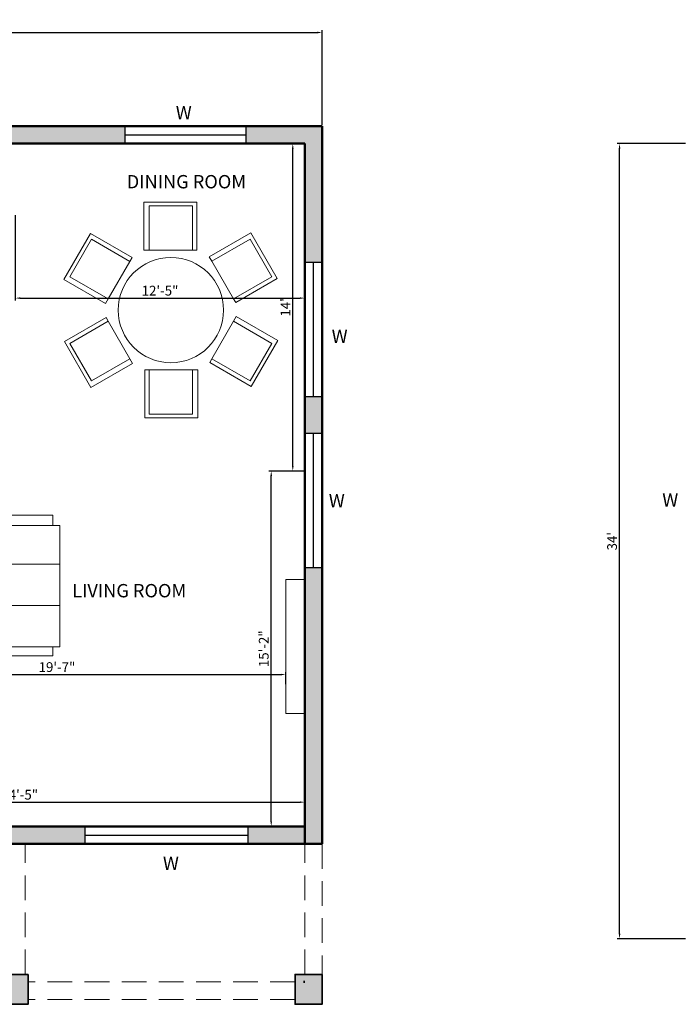
# Model space of a CAD drawing. Units: inches. Extents: x 1838 to 3464, y 573 to 2547.
# Tile 3 of 6: x 2449 to 2788, y 1302 to 1808. Entities that reach past the tile are written whole.
import ezdxf

# ---------------------------------------------------------------- set-up
doc = ezdxf.new("R2010")
doc.units = ezdxf.units.IN
doc.linetypes.add('DASHED', pattern=[19.05, 12.7, -6.35])
for name, color, linetype, lineweight in [('A-ANNO-DIMS', 2, 'Continuous', 18), ('A-ANNO-TEXT', 7, 'Continuous', 18), ('A-AREA-IDEN', 3, 'Continuous', 18), ('A-COLS', 6, 'Continuous', 35), ('A-FLOR-OVHD', 8, 'DASHED', 18), ('A-FURN', 8, 'Continuous', 18), ('A-GLAZ', 3, 'Continuous', 25), ('A-WALL', 1, 'Continuous', 50), ('A-WALL-PATT', 8, 'Continuous', 13)]:
    doc.layers.add(name, color=color, linetype=linetype, lineweight=lineweight)
doc.styles.get("Standard").update_dxf_attribs({"font": 'arial.ttf'})
doc.dimstyles.new('ISO-25', dxfattribs={"dimtxt": 5, "dimasz": 2.5, "dimexe": 1.25, "dimexo": 0.625, "dimtad": 1, "dimdec": 0, "dimlunit": 4, "dimtxsty": 'Standard', "dimcen": 2.5, "dimadec": 0, "dimazin": 0, "dimtfac": 1, "dimtdec": 0, "dimtmove": 0, "dimatfit": 3, "dimfxl": 1, "dimarcsym": 0})

# ---------------------------------------------------------------- blocks, each defined once
blk = doc.blocks.new('*U5')
for p, q in [((-13.85, 16.56), (-13.85, 41.18)), ((-13.85, 41.18), (13.34, 41.18)), ((13.34, 41.18), (13.34, 16.56)), ((-11.15, 16.56), (-13.85, 16.56)), ((13.34, 16.56), (11.13, 16.56))]:
    blk.add_line(p, q)
blk.add_lwpolyline([(-11.15, 16.56), (11.13, 16.56), (11.13, 39.27), (-11.15, 39.27)], close=True)
blk.add_circle((0, -14.18), 27.01)
blk = doc.blocks.new('*U6')
at = {"layer": 'A-FURN', "transparency": 16777216}
blk.add_blockref('*U5', (2526.78, 1672.86), dxfattribs=at)
for p, rotation in [((2514.5, 1665.77), 60), ((2539.06, 1665.77), 300), ((2514.5, 1651.59), 120), ((2539.06, 1651.59), 240), ((2526.78, 1644.5), 180)]:
    blk.add_blockref('*U5', p, dxfattribs=dict(at, rotation=rotation))
blk = doc.blocks.new('*D13')
at = {"layer": 'A-ANNO-DIMS', "color": 0, "lineweight": -2, "transparency": 16777216}
for p, q in [((2302.96, 1394.32), (2302.96, 1407.41)), ((2305.46, 1406.16), (2592.96, 1406.16)), ((2595.46, 1394.32), (2595.46, 1407.41))]:
    blk.add_line(p, q, dxfattribs=at)
at = {"layer": 'A-ANNO-DIMS', "color": 0, "lineweight": 100, "transparency": 16777216}
for points in [[(2305.46, 1406.58), (2305.46, 1405.75), (2302.96, 1406.16)], [(2592.96, 1406.58), (2592.96, 1405.75), (2595.46, 1406.16)]]:
    blk.add_solid(points, dxfattribs=at)
at = {"layer": 'Defpoints', "color": 0, "lineweight": 100, "transparency": 16777216}
for p in [(2595.46, 1406.16), (2302.96, 1393.69), (2595.46, 1393.69)]:
    blk.add_point(p, dxfattribs=at)
at = {"layer": 'A-ANNO-DIMS', "color": 0, "transparency": 16777216, "insert": (2449.21, 1409.34), "char_height": 5, "attachment_point": 5}
blk.add_mtext('24\'-5"', dxfattribs=at)
blk = doc.blocks.new('*D14')
at = {"layer": 'A-ANNO-DIMS', "color": 0, "lineweight": -2, "transparency": 16777216}
for p, q in [((2594.83, 1576.09), (2577.01, 1576.09)), ((2578.26, 1396.19), (2578.26, 1573.59)), ((2594.83, 1393.69), (2577.01, 1393.69))]:
    blk.add_line(p, q, dxfattribs=at)
at = {"layer": 'A-ANNO-DIMS', "color": 0, "lineweight": 100, "transparency": 16777216}
for points in [[(2577.85, 1573.59), (2578.68, 1573.59), (2578.26, 1576.09)], [(2577.85, 1396.19), (2578.68, 1396.19), (2578.26, 1393.69)]]:
    blk.add_solid(points, dxfattribs=at)
at = {"layer": 'Defpoints', "color": 0, "lineweight": 100, "transparency": 16777216}
for p in [(2578.26, 1576.09), (2595.46, 1576.09), (2595.46, 1393.69)]:
    blk.add_point(p, dxfattribs=at)
at = {"layer": 'A-ANNO-DIMS', "color": 0, "transparency": 16777216, "insert": (2575.08, 1484.89), "char_height": 5, "attachment_point": 5, "rotation": 90}
blk.add_mtext('15\'-2"', dxfattribs=at)
blk = doc.blocks.new('*D15')
at = {"layer": 'A-ANNO-DIMS', "color": 0, "lineweight": -2, "transparency": 16777216}
for p, q in [((2594.83, 1744.09), (2588.08, 1744.09)), ((2589.33, 1578.59), (2589.33, 1741.59)), ((2594.83, 1576.09), (2588.08, 1576.09))]:
    blk.add_line(p, q, dxfattribs=at)
at = {"layer": 'A-ANNO-DIMS', "color": 0, "lineweight": 100, "transparency": 16777216}
for points in [[(2588.91, 1741.59), (2589.74, 1741.59), (2589.33, 1744.09)], [(2588.91, 1578.59), (2589.74, 1578.59), (2589.33, 1576.09)]]:
    blk.add_solid(points, dxfattribs=at)
at = {"layer": 'Defpoints', "color": 0, "lineweight": 100, "transparency": 16777216}
for p in [(2589.33, 1744.09), (2595.46, 1744.09), (2595.46, 1576.09)]:
    blk.add_point(p, dxfattribs=at)
at = {"layer": 'A-ANNO-DIMS', "color": 0, "transparency": 16777216, "insert": (2586.19, 1660.09), "char_height": 5, "attachment_point": 5, "rotation": 90}
blk.add_mtext("14'", dxfattribs=at)
blk = doc.blocks.new('*D16')
at = {"layer": 'A-ANNO-DIMS', "color": 0, "lineweight": -2, "transparency": 16777216}
for p, q in [((2446.96, 1707.46), (2446.96, 1663.58)), ((2595.46, 1707.46), (2595.46, 1663.58)), ((2449.46, 1664.83), (2592.96, 1664.83))]:
    blk.add_line(p, q, dxfattribs=at)
at = {"layer": 'A-ANNO-DIMS', "color": 0, "lineweight": 100, "transparency": 16777216}
for points in [[(2449.46, 1665.25), (2449.46, 1664.41), (2446.96, 1664.83)], [(2592.96, 1665.25), (2592.96, 1664.41), (2595.46, 1664.83)]]:
    blk.add_solid(points, dxfattribs=at)
at = {"layer": 'Defpoints', "color": 0, "lineweight": 100, "transparency": 16777216}
for p in [(2446.96, 1708.09), (2595.46, 1708.09), (2595.46, 1664.83)]:
    blk.add_point(p, dxfattribs=at)
at = {"layer": 'A-ANNO-DIMS', "color": 0, "transparency": 16777216, "insert": (2521.21, 1668.01), "char_height": 5, "attachment_point": 5}
blk.add_mtext('12\'-5"', dxfattribs=at)
blk = doc.blocks.new('*D17')
at = {"layer": 'A-ANNO-DIMS', "color": 0, "lineweight": -2, "transparency": 16777216}
for p, q in [((2350.96, 1466.71), (2350.96, 1472.89)), ((2353.46, 1471.64), (2583.23, 1471.64)), ((2585.73, 1466.71), (2585.73, 1472.89))]:
    blk.add_line(p, q, dxfattribs=at)
at = {"layer": 'A-ANNO-DIMS', "color": 0, "lineweight": 100, "transparency": 16777216}
for points in [[(2353.46, 1472.06), (2353.46, 1471.23), (2350.96, 1471.64)], [(2583.23, 1472.06), (2583.23, 1471.23), (2585.73, 1471.64)]]:
    blk.add_solid(points, dxfattribs=at)
at = {"layer": 'Defpoints', "color": 0, "lineweight": 100, "transparency": 16777216}
for p in [(2585.73, 1471.64), (2350.96, 1466.09), (2585.73, 1466.09)]:
    blk.add_point(p, dxfattribs=at)
at = {"layer": 'A-ANNO-DIMS', "color": 0, "transparency": 16777216, "insert": (2468.34, 1474.82), "char_height": 5, "attachment_point": 5}
blk.add_mtext('19\'-7"', dxfattribs=at)
blk = doc.blocks.new('*D20')
at = {"layer": 'A-ANNO-DIMS', "color": 0, "lineweight": -2, "transparency": 16777216}
for p, q in [((2124.46, 1753.71), (2124.46, 1802.37)), ((2126.96, 1801.12), (2601.96, 1801.12)), ((2604.46, 1753.71), (2604.46, 1802.37))]:
    blk.add_line(p, q, dxfattribs=at)
at = {"layer": 'A-ANNO-DIMS', "color": 0, "lineweight": 100, "transparency": 16777216}
for points in [[(2126.96, 1801.54), (2126.96, 1800.7), (2124.46, 1801.12)], [(2601.96, 1801.54), (2601.96, 1800.7), (2604.46, 1801.12)]]:
    blk.add_solid(points, dxfattribs=at)
at = {"layer": 'Defpoints', "color": 0, "lineweight": 100, "transparency": 16777216}
for p in [(2604.46, 1801.12), (2124.46, 1753.09), (2604.46, 1753.09)]:
    blk.add_point(p, dxfattribs=at)
at = {"layer": 'A-ANNO-DIMS', "color": 0, "transparency": 16777216, "insert": (2364.46, 1804.3), "char_height": 5, "attachment_point": 5}
blk.add_mtext("40'", dxfattribs=at)
blk = doc.blocks.new('*D66')
at = {"layer": 'A-ANNO-DIMS', "color": 0, "lineweight": -2, "transparency": 16777216}
for p, q in [((2790.9, 1744.09), (2755.73, 1744.09)), ((2756.98, 1338.59), (2756.98, 1741.59)), ((2790.9, 1336.09), (2755.73, 1336.09))]:
    blk.add_line(p, q, dxfattribs=at)
at = {"layer": 'A-ANNO-DIMS', "color": 0, "lineweight": 100, "transparency": 16777216}
for points in [[(2756.56, 1741.59), (2757.39, 1741.59), (2756.98, 1744.09)], [(2756.56, 1338.59), (2757.39, 1338.59), (2756.98, 1336.09)]]:
    blk.add_solid(points, dxfattribs=at)
at = {"layer": 'Defpoints', "color": 0, "lineweight": 100, "transparency": 16777216}
for p in [(2756.98, 1744.09), (2791.52, 1744.09), (2791.52, 1336.09)]:
    blk.add_point(p, dxfattribs=at)
at = {"layer": 'A-ANNO-DIMS', "color": 0, "transparency": 16777216, "insert": (2753.8, 1540.09), "char_height": 5, "attachment_point": 5, "rotation": 90}
blk.add_mtext("34'", dxfattribs=at)

msp = doc.modelspace()

# ---------------------------------------------------------------- hatches: boundary and pattern name
at = {"layer": 'A-WALL-PATT'}
h = msp.add_hatch(color=256, dxfattribs=at)
h.dxf.hatch_style = 1
h.paths.add_polyline_path([(2238.51, 1753.09), (2124.46, 1753.09), (2124.46, 1570.41), (2133.46, 1570.41), (2133.46, 1606.09), (2133.46, 1744.09), (2238.51, 1744.09)])
h.paths.add_polyline_path([(2351.42, 1753.09), (2279.74, 1753.09), (2279.74, 1744.09), (2351.42, 1744.09)])
h.paths.add_polyline_path([(2503.16, 1753.09), (2416.24, 1753.09), (2416.24, 1744.09), (2446.96, 1744.09), (2503.16, 1744.09)])
h.paths.add_polyline_path([(2604.46, 1753.09), (2565.42, 1753.09), (2565.42, 1744.09), (2595.46, 1744.09), (2595.46, 1683.21), (2604.46, 1683.21)])
h.paths.add_polyline_path([(2133.46, 1501.38), (2124.46, 1501.38), (2124.46, 1354.09), (2133.46, 1354.09)])
h.paths.add_polyline_path([(2291.43, 1354.09), (2135.98, 1354.09), (2135.98, 1345.09), (2291.43, 1345.09)])
h.paths.add_polyline_path([(2321.13, 1390.69), (2321.13, 1393.69), (2302.96, 1393.69), (2302.96, 1384.69), (2321.13, 1384.69)])
h.paths.add_polyline_path([(2482.67, 1393.69), (2361.02, 1393.69, -0.01877), (2361.13, 1390.69), (2361.13, 1384.69), (2482.67, 1384.69)])
h.paths.add_polyline_path([(2302.96, 1576.09), (2302.96, 1610.48), (2302.96, 1744.09), (2298.46, 1744.09), (2298.46, 1571.59), (2298.46, 1354.09), (2302.96, 1354.09)])
h.paths.add_polyline_path([(2595.46, 1393.69), (2566.49, 1393.69), (2566.49, 1384.69), (2595.46, 1384.69)])
h.paths.add_polyline_path([(2604.46, 1526.49), (2595.46, 1526.49), (2595.46, 1404.09), (2595.46, 1384.69), (2604.46, 1384.69)])
h.paths.add_polyline_path([(2604.46, 1614.19), (2595.46, 1614.19), (2595.46, 1595.51), (2604.46, 1595.51)])
h = msp.add_hatch(color=256, dxfattribs=at)
h.dxf.hatch_style = 1
h.paths.add_polyline_path([(2135.98, 1354.09), (2124.46, 1354.09), (2124.46, 1342.67), (2135.98, 1342.67)])
h.paths.add_polyline_path([(2302.96, 1354.09), (2291.43, 1354.09), (2291.43, 1342.67), (2302.96, 1342.67)])
h.paths.add_polyline_path([(2453.5, 1317.8), (2439.65, 1317.8), (2439.65, 1302.42), (2453.5, 1302.42)])
h.paths.add_polyline_path([(2302.96, 1317.8), (2289.1, 1317.8), (2289.1, 1302.42), (2302.96, 1302.42)])
h.paths.add_polyline_path([(2604.33, 1317.8), (2590.48, 1317.8), (2590.48, 1302.42), (2604.33, 1302.42)])

# ---------------------------------------------------------------- linework, layer by layer
at = {"layer": 'A-COLS'}
for points in [[(2453.5, 1317.8), (2439.65, 1317.8), (2439.65, 1302.42), (2453.5, 1302.42)], [(2604.33, 1317.8), (2590.48, 1317.8), (2590.48, 1302.42), (2604.33, 1302.42)]]:
    msp.add_lwpolyline(points, close=True, dxfattribs=at)
at = {"layer": 'A-FLOR-OVHD'}
for p, q in [((2452, 1317.8), (2452, 1384.69)), ((2595.46, 1317.8), (2595.46, 1384.69)), ((2604.46, 1384.69), (2604.33, 1317.8)), ((2590.48, 1313.93), (2453.5, 1313.93)), ((2590.48, 1304.93), (2453.5, 1304.93))]:
    msp.add_line(p, q, dxfattribs=at)
at = {"layer": 'A-FURN'}
for p, q in [((2441.01, 1553.46), (2466.28, 1553.46)), ((2466.28, 1553.46), (2466.28, 1548.22)), ((2469.8, 1528.32), (2444.27, 1528.32)), ((2469.8, 1507.14), (2444.27, 1507.14)), ((2466.28, 1485.82), (2466.28, 1481.22)), ((2466.28, 1481.22), (2441.01, 1481.22))]:
    msp.add_line(p, q, dxfattribs=at)
for points in [[(2469.8, 1548.22), (2444.27, 1548.22), (2444.27, 1485.82), (2469.8, 1485.82)], [(2595.46, 1451.67), (2585.73, 1451.67), (2585.73, 1520.47), (2595.46, 1520.47)]]:
    msp.add_lwpolyline(points, close=True, dxfattribs=at)
at = {"layer": 'A-GLAZ'}
for p, q in [((2503.16, 1748.59), (2565.42, 1748.59)), ((2599.96, 1614.19), (2599.96, 1683.21)), ((2599.96, 1526.49), (2599.96, 1595.51)), ((2482.67, 1389.19), (2566.49, 1389.19))]:
    msp.add_line(p, q, dxfattribs=at)
for points in [[(2503.16, 1744.09), (2565.42, 1744.09), (2565.42, 1753.09), (2503.16, 1753.09)], [(2595.46, 1683.21), (2604.46, 1683.21), (2604.46, 1614.19), (2595.46, 1614.19)], [(2595.46, 1595.51), (2604.46, 1595.51), (2604.46, 1526.49), (2595.46, 1526.49)], [(2482.67, 1384.69), (2566.49, 1384.69), (2566.49, 1393.69), (2482.67, 1393.69)]]:
    msp.add_lwpolyline(points, close=True, dxfattribs=at)
at = {"layer": 'A-WALL'}
for p, q in [((2124.46, 1753.09), (2604.46, 1753.09)), ((2604.46, 1753.09), (2604.46, 1384.69)), ((2133.46, 1744.09), (2595.46, 1744.09)), ((2595.46, 1744.09), (2451.46, 1744.09)), ((2595.46, 1744.09), (2595.46, 1384.69)), ((2595.46, 1744.09), (2595.46, 1404.09)), ((2595.46, 1404.09), (2595.46, 1384.69)), ((2595.46, 1393.69), (2361.02, 1393.69)), ((2595.46, 1384.69), (2361.13, 1384.69)), ((2595.46, 1384.69), (2604.46, 1384.69)), ((2594.74, 1313.93), (2595.46, 1313.93))]:
    msp.add_line(p, q, dxfattribs=at)

# ---------------------------------------------------------------- block references
at = {"layer": 'A-FURN'}
msp.add_blockref('*U6', (0, 0), dxfattribs=at)

# ---------------------------------------------------------------- texts
at = {"layer": 'A-ANNO-TEXT', "char_height": 6.84, "attachment_point": 1}
for insert in [(2529.28, 1763.47), (2609.27, 1648.7), (2607.8, 1564.29), (2778.9, 1564.65), (2522.69, 1378.24)]:
    msp.add_mtext_dynamic_manual_height_columns('W', width=95.5762, gutter_width=34.2, heights=[0], dxfattribs=dict(at, insert=insert))
at = {"layer": 'A-AREA-IDEN', "char_height": 6.8407, "attachment_point": 1}
for s, insert in [('DINING ROOM', (2504.11, 1727.99)), ('LIVING ROOM', (2476.14, 1518.11))]:
    msp.add_mtext_dynamic_manual_height_columns(s, width=95.5762, gutter_width=34.2, heights=[0], dxfattribs=dict(at, insert=insert))

# ---------------------------------------------------------------- dimensions: what is measured, and where the dimension line sits
at = {"layer": 'A-ANNO-DIMS'}
for base, p1, p2, picture, middle in [((2604.46, 1801.12), (2124.46, 1753.09), (2604.46, 1753.09), '*D20', (2364.46, 1804.3)), ((2595.45522311, 1664.82921857), (2446.95522311, 1708.08520436), (2595.45522311, 1708.08520436), '*D16', (2521.20522311, 1668.00708351)), ((2585.73, 1471.64), (2350.96, 1466.09), (2585.73, 1466.09), '*D17', (2468.34, 1474.82)), ((2595.45522311, 1406.16307805), (2302.95522311, 1393.69353478), (2595.45522311, 1393.69353478), '*D13', (2449.20522311, 1409.34094299))]:
    dim = msp.add_linear_dim(base=base, p1=p1, p2=p2, dimstyle='ISO-25', override={"dimclrd": 0, "dimclre": 0, "dimclrt": 0}, dxfattribs=at)
    dim.commit()
    dim.dimension.update_dxf_attribs({"geometry": picture, "text_midpoint": middle})
for base, p1, p2, picture, middle in [((2589.33, 1744.09), (2595.46, 1576.09), (2595.46, 1744.09), '*D15', (2586.19, 1660.09)), ((2756.98, 1744.09), (2791.52, 1336.09), (2791.52, 1744.09), '*D66', (2753.8, 1540.09)), ((2578.26, 1576.09), (2595.46, 1393.69), (2595.46, 1576.09), '*D14', (2575.08, 1484.89))]:
    dim = msp.add_linear_dim(base=base, p1=p1, p2=p2, angle=90, dimstyle='ISO-25', override={"dimclrd": 0, "dimclre": 0, "dimclrt": 0}, dxfattribs=at)
    dim.commit()
    dim.dimension.update_dxf_attribs({"geometry": picture, "text_midpoint": middle})

doc.saveas('drawing.dxf')
